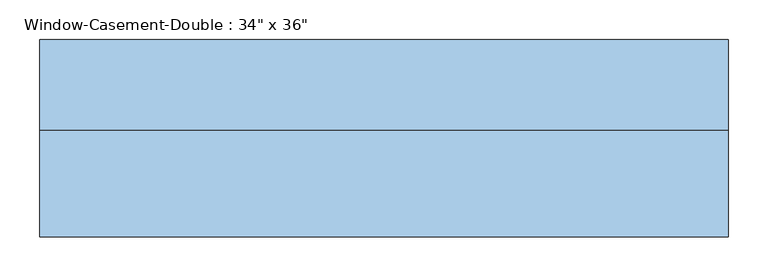
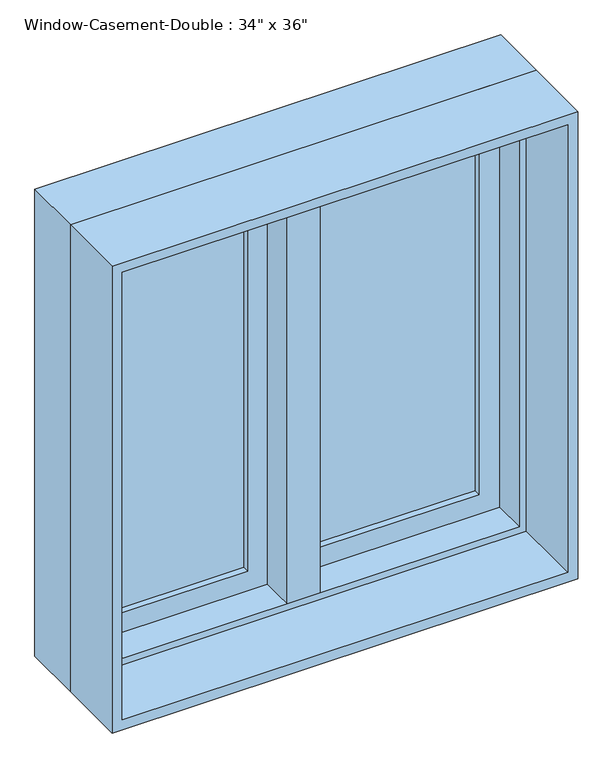
"""IFC4 building model written with IfcOpenShell, lengths in millimetres: window geometry."""

from ifc_helpers import new_model, si_unit, frame, origin, place, context, project, spatial, polyline, outline, extrude, faceted_brep, source, transform, mapped, element, save


def window_339605e1(model_context):
    return source(origin(), model_context, "Body", "SolidModel", [
        faceted_brep([(9.525, 133.35, 1816.1), (-9.525, 133.35, 1816.1), (-9.525, 82.55, 1816.1), (9.525, 82.55, 1816.1), (9.525, 133.35, 927.1), (9.525, 82.55, 927.1), (-9.525, 82.55, 927.1), (-9.525, 133.35, 927.1), (-9.525, 82.55, 946.15), (-9.525, 82.55, 1797.05), (-30.1625, 82.55, 946.15), (-30.1625, 82.55, 1797.05), (-30.1625, 19.05, 946.15), (-30.1625, 19.05, 1797.05), (30.1625, 19.05, 946.15), (30.1625, 19.05, 1797.05), (30.1625, 82.55, 946.15), (30.1625, 82.55, 1797.05), (9.525, 82.55, 946.15), (9.525, 82.55, 1797.05)], [[[0, 1, 2, 3]], [[4, 5, 6, 7]], [[1, 0, 4, 7]], [[2, 1, 7, 6, 8, 9]], [[9, 8, 10, 11]], [[11, 10, 12, 13]], [[13, 12, 14, 15]], [[15, 14, 16, 17]], [[17, 16, 18, 19]], [[0, 3, 19, 18, 5, 4]], [[18, 8, 6, 5]], [[9, 19, 3, 2]], [[8, 18, 16, 14, 12, 10]], [[19, 9, 11, 13, 15, 17]]]),
        extrude(outline(polyline([(-66.675, 114.3), (-66.675, 107.95), (-361.95, 107.95), (-361.95, 114.3), (-66.675, 114.3)])), frame((0.0, 0.0, 984.25), z_axis=(0.0, 0.0, 1.0), x_axis=(1.0, 0.0, 0.0)), (0.0, 0.0, 1.0), 774.7),
        extrude(outline(polyline([(-361.95, 95.25), (-361.95, 101.6), (-66.675, 101.6), (-66.675, 95.25), (-361.95, 95.25)])), frame((0.0, 0.0, 984.25), z_axis=(0.0, 0.0, 1.0), x_axis=(1.0, 0.0, 0.0)), (0.0, 0.0, 1.0), 774.7),
        extrude(outline(polyline([(361.95, 114.3), (361.95, 107.95), (66.675, 107.95), (66.675, 114.3), (361.95, 114.3)])), frame((0.0, 0.0, 984.25), z_axis=(0.0, 0.0, 1.0), x_axis=(1.0, 0.0, 0.0)), (0.0, 0.0, 1.0), 774.7),
        extrude(outline(polyline([(66.675, 95.25), (66.675, 101.6), (361.95, 101.6), (361.95, 95.25), (66.675, 95.25)])), frame((0.0, 0.0, 984.25), z_axis=(0.0, 0.0, 1.0), x_axis=(1.0, 0.0, 0.0)), (0.0, 0.0, 1.0), 774.7),
        extrude(outline(polyline([(1816.1, -419.1), (927.1, -419.1), (927.1, -9.525), (1816.1, -9.525), (1816.1, -419.1)]), holes=[polyline([(1758.95, -66.675), (984.25, -66.675), (984.25, -361.95), (1758.95, -361.95), (1758.95, -66.675)])]), frame((0.0, 82.55, 0.0), z_axis=(0.0, 1.0, 0.0), x_axis=(0.0, 0.0, 1.0)), (0.0, 0.0, 1.0), 44.45),
        extrude(outline(polyline([(927.1, 419.1), (1816.1, 419.1), (1816.1, 9.525), (927.1, 9.525), (927.1, 419.1)]), holes=[polyline([(984.25, 66.675), (1758.95, 66.675), (1758.95, 361.95), (984.25, 361.95), (984.25, 66.675)])]), frame((0.0, 82.55, 0.0), z_axis=(0.0, 1.0, 0.0), x_axis=(0.0, 0.0, 1.0)), (0.0, 0.0, 1.0), 44.45),
        extrude(outline(polyline([(1828.8, -431.8), (914.4, -431.8), (914.4, 431.8), (1828.8, 431.8), (1828.8, -431.8)]), holes=[polyline([(1809.75, 412.75), (933.45, 412.75), (933.45, -412.75), (1809.75, -412.75), (1809.75, 412.75)])]), frame((0.0, -114.3, 0.0), z_axis=(0.0, 1.0, 0.0), x_axis=(0.0, 0.0, 1.0)), (0.0, 0.0, 1.0), 133.35),
        faceted_brep([(400.05, 82.55, 1797.05), (400.05, 19.05, 1797.05), (-400.05, 19.05, 1797.05), (-400.05, 82.55, 1797.05), (419.1, 133.35, 1816.1), (419.1, 82.55, 1816.1), (-419.1, 82.55, 1816.1), (-419.1, 133.35, 1816.1), (431.8, 19.05, 1828.8), (431.8, 133.35, 1828.8), (-431.8, 133.35, 1828.8), (-431.8, 19.05, 1828.8), (-400.05, 19.05, 946.15), (-400.05, 82.55, 946.15), (-419.1, 82.55, 927.1), (-419.1, 133.35, 927.1), (-431.8, 133.35, 914.4), (-431.8, 19.05, 914.4), (400.05, 19.05, 946.15), (400.05, 82.55, 946.15), (419.1, 82.55, 927.1), (419.1, 133.35, 927.1), (431.8, 133.35, 914.4), (431.8, 19.05, 914.4)], [[[0, 1, 2, 3]], [[4, 5, 6, 7]], [[8, 9, 10, 11]], [[3, 2, 12, 13]], [[7, 6, 14, 15]], [[11, 10, 16, 17]], [[13, 12, 18, 19]], [[15, 14, 20, 21]], [[17, 16, 22, 23]], [[11, 17, 23, 8], [1, 18, 12, 2]], [[19, 18, 1, 0]], [[5, 20, 14, 6], [3, 13, 19, 0]], [[21, 20, 5, 4]], [[23, 22, 9, 8]], [[9, 22, 16, 10], [7, 15, 21, 4]]]),
    ])


if __name__ == "__main__":
    model = new_model("IFC4")
    model_context = context("Model", 3, world=origin())
    ifc_project = project(units=[si_unit("LENGTHUNIT", "METRE", prefix="MILLI")], contexts=[model_context])
    site = spatial("IfcSite", under=ifc_project)
    building = spatial("IfcBuilding", under=site)
    placement = place(None, origin())
    window_shape = window_339605e1(model_context)
    element("IfcWindow", 1, ObjectType="Window-Casement-Double : 34\" x 36\"", at=placement, inside=building, context=model_context, shape_type="MappedRepresentation", body=[
        mapped(window_shape, transform((0.0, 0.0, 0.0), x_axis=(1.0, 0.0, 0.0), y_axis=(0.0, 1.0, 0.0), z_axis=(0.0, 0.0, 1.0))),
    ])
    save(model, "model.ifc")

# Revit data of these elements
# Type "Window-Casement-Double : 34\" x 36\""
#   Type Mark = "14"
#   Fire Rating = "0.5h"
#   Assembly Code = "B2020100"
#   Analytic Construction = "Double glazing - domestic"
#   Frame Extension [instance default] = 0.020833 ft
#   Window Inset [instance default] = 0 ft
#   Wall Thickness [instance default] = 0.5 ft
#   Interior Wall Closure [instance default] = 0.1875 ft
#   Half Width = 1.416667 ft
#   Visual Light Transmittance = 0.81
#   Thermal Resistance (R) = 1.8146 (h·ft²·°F)/BTU
#   Solar Heat Gain Coefficient = 0.76
#   Rough Width = 2.875 ft
#   Rough Height = 3.041667 ft
#   Height = 3 ft
#   Heat Transfer Coefficient (U) = 0.5511 BTU/(h·ft²·°F)
#   Exterior Wall Closure [instance default] = 0.104167 ft
#   Extension Jamb [instance default] = 0.1875 ft
#   Default Sill Height = 3 ft
#   Width = 2.833333 ft
#   Define Thermal Properties by = 0
#   Muntin Visibility = yes
#   Interior Trim Visibility [instance default] = yes
#   Exterior Trim Visibility [instance default] = yes
#   Extension Jamb Visibility [instance default] = yes
#   Interior Trim Material = Wood - Stained
#   Muntin Pattern = Muntin Pattern_2x2 : Muntin Pattern_2x2
#   Interior Trim = Trim-Window-Interior-Flat : Picture Frame
#   Interior Frame Material = Wood - Stained
#   Glass Panel Material = Glass
#   Exterior Trim Material = Clad - White
#   Exterior Trim = Trim-Window-Exterior-Flat : with Sill
#   Exterior Frame Material = Clad - White
#   Wall Closure = (empty or 0)
# Element 1 (IfcWindow, "Window-Casement-Double : 34\" x 36\"")
#   Wall Thickness = 0.75 ft
#   Extension Jamb = 0.4375 ft
#   Materials on its faces: "Wood - Stained", "Glass", "Clad - White"
# Materials
#   "Wood - Stained": class "Wood", colour RGB 224 178 126, transparency 0, Cost = 0
#   "Glass": class "Glass", colour RGB 0 128 192, transparency 0.75, Description = "Soda Lime Glass", Cost = 0
#   "Clad - White": class "Wood", colour RGB 242 242 238, transparency 0, Cost = 0
